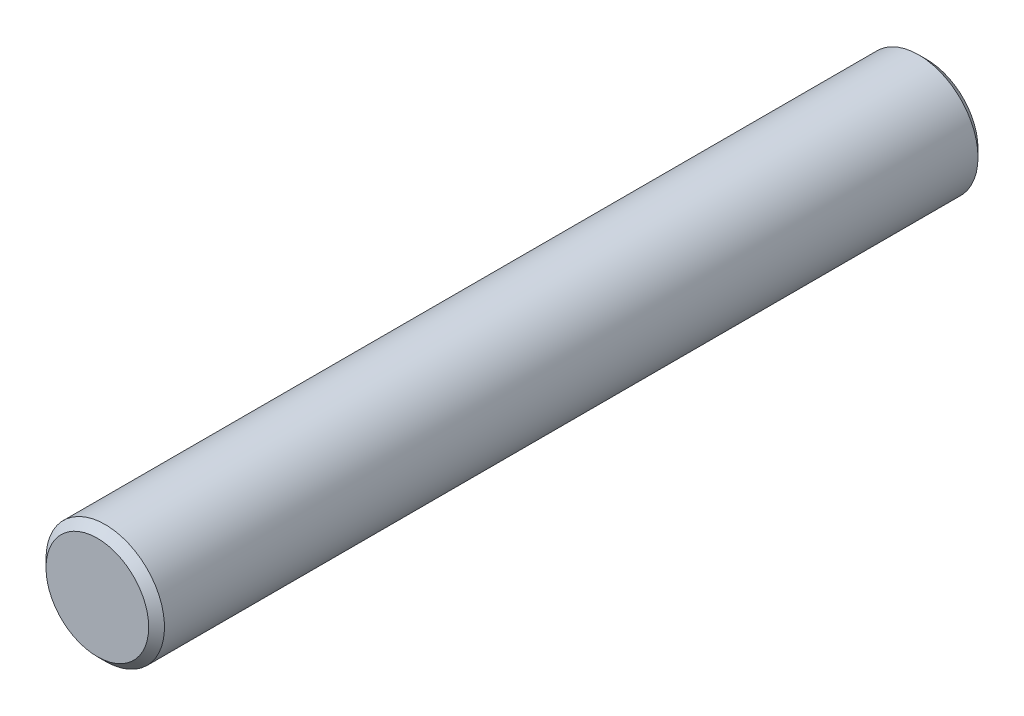
SolidWorks part; units mm, degrees
material "Plain Carbon Steel"
ref_plane "Front Plane" through (0, 0, 0) normal (0, 0, 1) x (1, 0, 0)
ref_plane "Top Plane" through (0, 0, 0) normal (0, 1, 0) x (1, 0, 0)
ref_plane "Right Plane" through (0, 0, 0) normal (1, 0, 0) x (0, 0, -1)
sketch "Pin Profile Ø3" plane through (0, 0, 0) normal (0, 0, 1) x (1, 0, 0)
  circle A0 centre (0, 0) radius 1.5
  dimension "D1" = 3
extrude "Pin Body Ø3x21" add sketch "Pin Profile Ø3" along normal mid plane 21
chamfer "End Chamfers 0.2x45°" distance 0.2 angle 45 2 edges at (1.5, 0, -10.5) (1.5, 0, 10.5)
